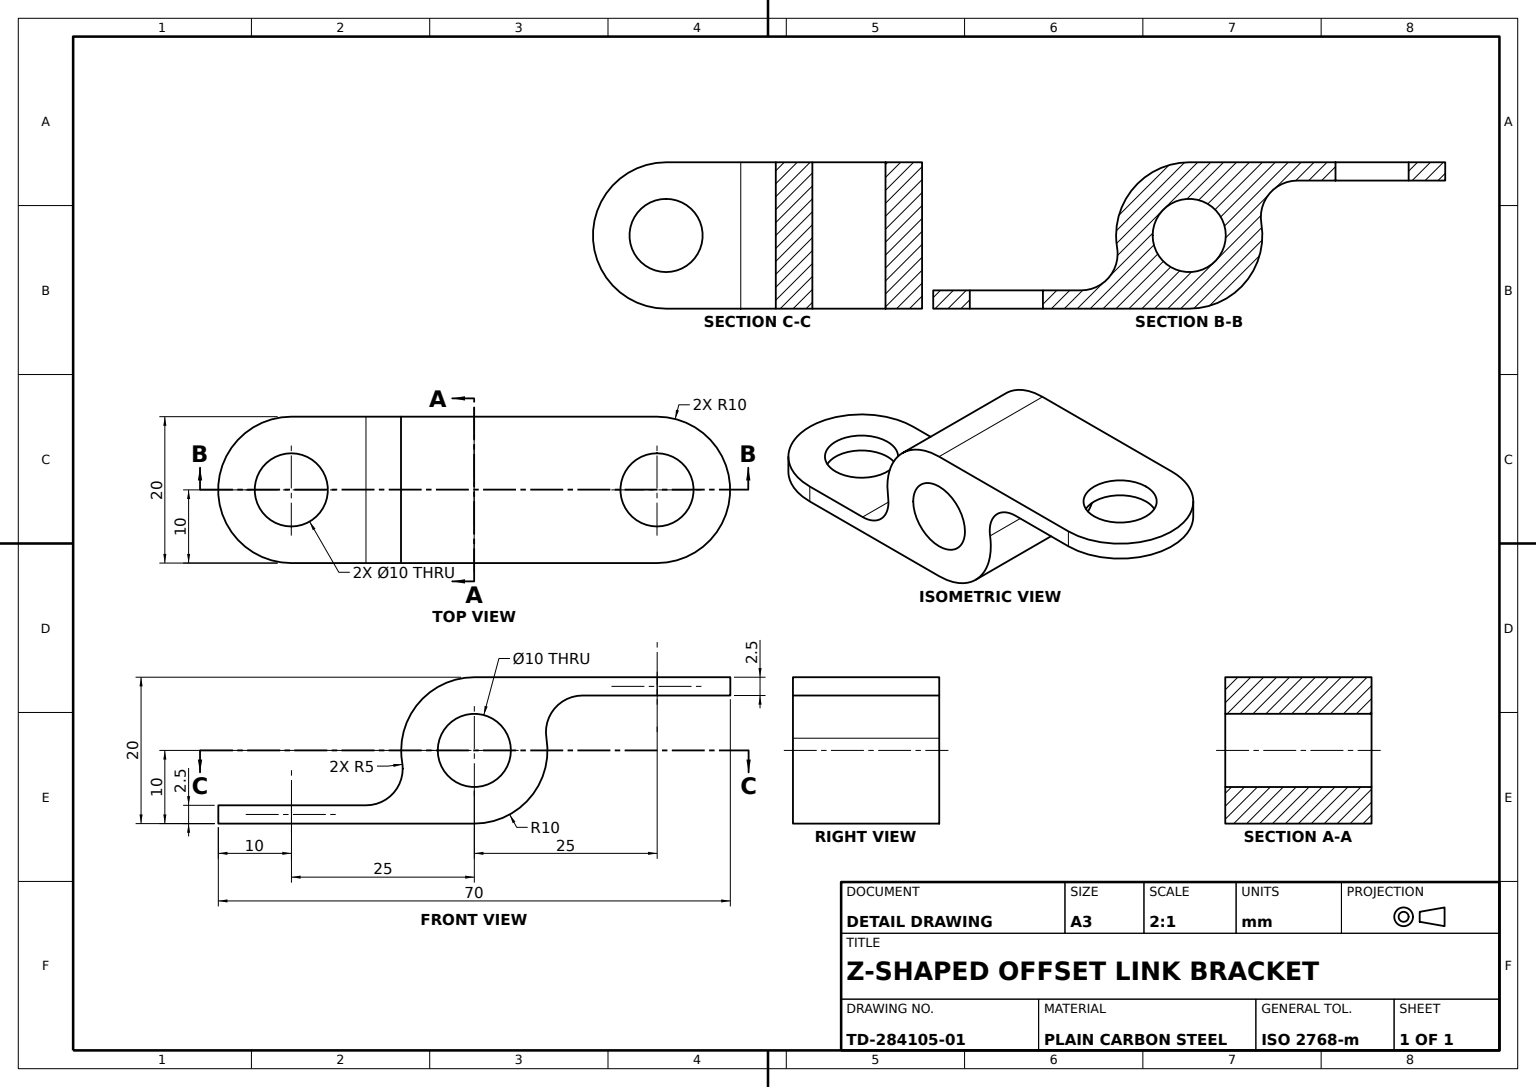
from build123d import *

# Parameters (mm, degrees)
HUB_SKETCH_20_R            = 10
HUB_CYLINDER_20_DEPTH      = 20
FIRST_START                = -20
FIRST_ARM_DEPTH            = 20
SECOND_START               = -20
SECOND_ARM_DEPTH           = 20
TAB_A_DEPTH                = 2.5
TAB_B_DEPTH                = 2.5
TAB_B_HOLE_SKETCH_10_R     = 5
TAB_B_HOLE_10_DEPTH        = 2.5
TAB_A_HOLE_SKETCH_10_R     = 5
TAB_A_HOLE_10_DEPTH        = 2.5
HUB_CROSS_BORE_SKETCH_10_R = 5
HUB_CROSS_BORE_10_DEPTH    = 20


with BuildPart() as part:
    # Hub Sketch Ø20 → Hub Cylinder Ø20 (new body)
    with BuildSketch(Plane.XY):
        Circle(HUB_SKETCH_20_R)
    extrude(amount=HUB_CYLINDER_20_DEPTH)

    # First Arm Sketch → First Arm (add)
    with BuildSketch(Plane.XY.offset(20).offset(FIRST_START)):
        with BuildLine():
            Line((0, 10), (25, 10))
            Line((25, 10), (25, 7.5))
            Line((25, 7.5), (6.614378278, 7.5))
            ThreePointArc((6.614378278, 7.5), (3.535533906, 9.354143467), (0, 10))
        make_face()
        with BuildLine():
            Line((0, -10), (-25, -10))
            Line((-25, -10), (-25, -7.5))
            Line((-25, -7.5), (-6.614378278, -7.5))
            ThreePointArc((-6.614378278, -7.5), (-3.535533906, -9.354143467), (0, -10))
        make_face()
    extrude(amount=FIRST_ARM_DEPTH)

    # Second Arm Sketch → Second Arm (add)
    with BuildSketch(Plane.XY.offset(20).offset(SECOND_START)):
        with BuildLine():
            ThreePointArc((-9.860132972, -1.666666667), (-10.971386379, -5.727486122), (-14.790199458, -7.5))
            Line((-14.790199458, -7.5), (-6.614378278, -7.5))
            ThreePointArc((-6.614378278, -7.5), (-8.738382269, -4.86216776), (-9.860132972, -1.666666667))
        make_face()
        with BuildLine():
            ThreePointArc((9.860132972, 1.666666667), (10.971386379, 5.727486122), (14.790199458, 7.5))
            Line((14.790199458, 7.5), (6.614378278, 7.5))
            ThreePointArc((6.614378278, 7.5), (8.738382269, 4.86216776), (9.860132972, 1.666666667))
        make_face()
    extrude(amount=SECOND_ARM_DEPTH)

    # Tab A Sketch → Tab A (add)
    with BuildSketch(Plane.XZ.offset(10)):
        with BuildLine():
            Line((-25, 20), (-25, 0))
            ThreePointArc((-25, 0), (-35, 10), (-25, 20))
        make_face()
    extrude(amount=-TAB_A_DEPTH)

    # Tab B Sketch → Tab B (add)
    with BuildSketch(Plane(origin=(0, 10, 0), x_dir=(1, 0, 0), z_dir=(0, 1, 0))):
        with BuildLine():
            Line((25, 0), (25, -20))
            ThreePointArc((25, -20), (35, -10), (25, 0))
        make_face()
    extrude(amount=-TAB_B_DEPTH)

    # Tab B Hole Sketch Ø10 → Tab B Hole Ø10 (cut)
    with BuildSketch(Plane(origin=(0, 10, 0), x_dir=(1, 0, 0), z_dir=(0, 1, 0))):
        with Locations(Location((25, -10, 0), (0, 0, 270))):
            Circle(TAB_B_HOLE_SKETCH_10_R)
    extrude(amount=-TAB_B_HOLE_10_DEPTH, mode=Mode.SUBTRACT)

    # Tab A Hole Sketch Ø10 → Tab A Hole Ø10 (cut)
    with BuildSketch(Plane.XZ.offset(10)):
        with Locations(Location((-25, 10, 0), (0, 0, 270))):
            Circle(TAB_A_HOLE_SKETCH_10_R)
    extrude(amount=-TAB_A_HOLE_10_DEPTH, mode=Mode.SUBTRACT)

    # Hub Cross Bore Sketch Ø10 → Hub Cross Bore Ø10 (cut)
    with BuildSketch(Plane.XY.offset(20)):
        Circle(HUB_CROSS_BORE_SKETCH_10_R)
    extrude(amount=-HUB_CROSS_BORE_10_DEPTH, mode=Mode.SUBTRACT)


solid = part.part
